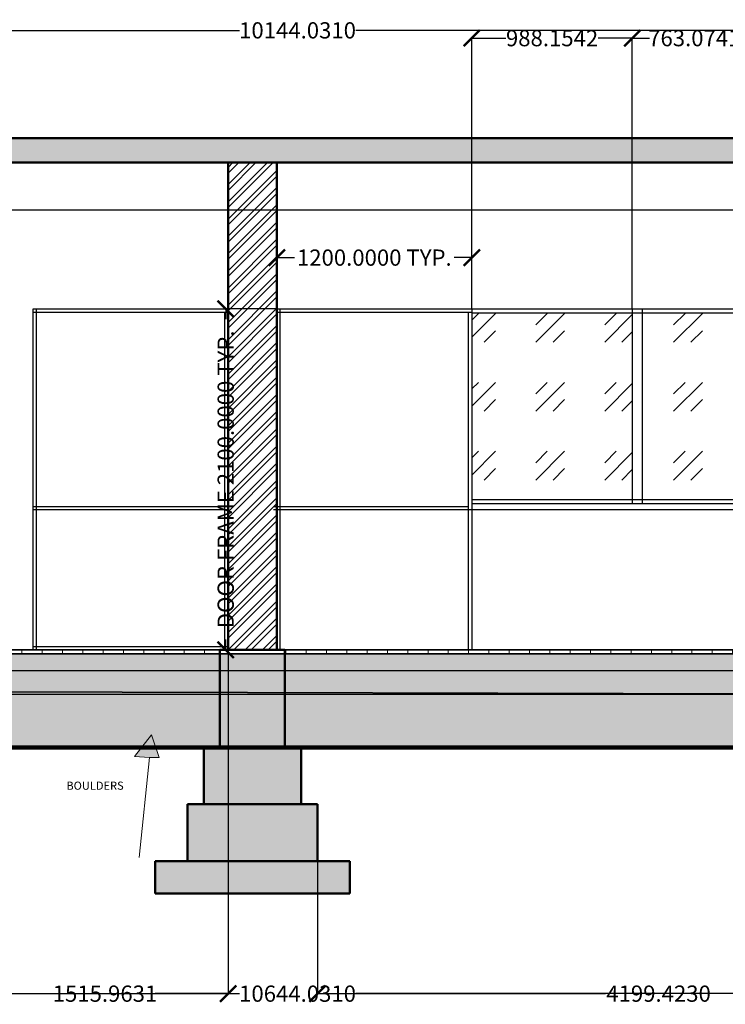
# Model space of a CAD drawing. Units: millimetres. Extents: x -4055 to 12299, y -682 to 5380.
# Tile 2 of 4: x 3612 to 7955, y -682 to 5380. Entities that reach past the tile are written whole.
import ezdxf

# ---------------------------------------------------------------- set-up
doc = ezdxf.new("R2010")
doc.units = ezdxf.units.MM
doc.header["$MEASUREMENT"] = 0
for name, color, linetype, lineweight in [('A-ANNO-DIMS', 2, 'Continuous', 18), ('A-ANNO-SYMB', 18, 'Continuous', 18), ('A-ANNO-TEXT', 7, 'Continuous', 18), ('A-DOOR', 3, 'Continuous', 25), ('A-FLOR', 7, 'Continuous', 35), ('A-FLOR-PATT', 8, 'Continuous', 13), ('A-GLAZ', 4, 'Continuous', 25), ('A-GLAZ-PATT', 8, 'Continuous', 13), ('A-ROOF', 7, 'Continuous', 50), ('A-ROOF-PATT', 8, 'Continuous', 13), ('A-WALL', 7, 'Continuous', 50), ('A-WALL-PATT', 8, 'Continuous', 13), ('gl', 18, 'Continuous', 120), ('S-FNDN', 7, 'Continuous', 50), ('S-FNDN-PATT', 8, 'Continuous', 13)]:
    doc.layers.add(name, color=color, linetype=linetype, lineweight=lineweight)
doc.styles.get("Standard").update_dxf_attribs({"font": 'arial.ttf'})
doc.dimstyles.get("Standard").update_dxf_attribs({"dimtxt": 100, "dimasz": 100, "dimexe": 0.18, "dimexo": 0.0625, "dimgap": 0.09, "dimtad": 0, "dimdec": 4, "dimzin": 0, "dimdsep": 46, "dimtxsty": 'Standard', "dimblk": 'ARCHTICK', "dimcen": 0.09, "dimclrd": 3, "dimclre": 6, "dimclrt": 1, "dimadec": 0, "dimazin": 0, "dimtfac": 1, "dimtdec": 4, "dimtofl": 0, "dimtmove": 0, "dimatfit": 3, "dimfxl": 1, "dimtolj": 1, "dimtzin": 0, "dimlwd": 30, "dimarcsym": 0})
pattern_1 = [(50, (0, 0), (71.72602, -6.2752), [7.5, -82.5]), (355, (0, 0), (-13.87513, 75.2192), [6, -66]), (100.45144, (5.98, -0.52), (57.8509, 68.944), [6.374, -70.1142]), (46.1842, (0, 20), (106.7241, -16.5519), [11.25, -123.75]), (96.6356, (8.89, 18.62), (93.4662, 97.4119), [9.561, -105.1714]), (351.1842, (0, 20), (93.4662, 97.4119), [9, -99]), (21, (10, 15), (59.6907, -40.2619), [7.5, -82.5]), (326, (10, 15), (24.33153, 72.515), [6, -66]), (71.45144, (14.974, 11.645), (84.02224, 32.2531), [6.374, -70.1142]), (37.5, (0, 0), (1.215986, 33.289385), [0, -65.2, 0, -67, 0, -66.25]), (7.5, (0, 0), (26.30695, 39.44117), [0, -38.2, 0, -63.7, 0, -25.25]), (327.5, (-22.3, 0), (53.382244, -2.25549), [0, -25, 0, -78, 0, -103.5]), (317.5, (-32.3, 0), (58.31862, 10.0105), [0, -32.5, 0, -51.8, 0, -73.5])]

# ---------------------------------------------------------------- blocks, each defined once
blk = doc.blocks.new('_ArchTick')
at = {"color": 0, "linetype": 'ByBlock', "const_width": 0.15}
blk.add_lwpolyline([(-0.5, -0.5), (0.5, 0.5)], dxfattribs=at)
blk = doc.blocks.new('*D12')
at = {"layer": 'A-ANNO-DIMS', "color": 0, "lineweight": -2, "transparency": 16777216}
for p, q in [((250, 4650.1), (250, 5314.3)), ((10394, 4650.1), (10394, 5314.3))]:
    blk.add_line(p, q, dxfattribs=at)
at = {"layer": 'A-ANNO-DIMS', "color": 0, "lineweight": 30, "transparency": 16777216}
for p, q in [((250, 5314.1), (4963.8, 5314.1)), ((10394, 5314.1), (5680.2, 5314.1))]:
    blk.add_line(p, q, dxfattribs=at)
at = {"layer": 'Defpoints', "color": 0, "transparency": 16777216}
for p in [(250, 5314.1), (250, 4650), (10394, 4650)]:
    blk.add_point(p, dxfattribs=at)
at = {"layer": 'A-ANNO-DIMS', "color": 0, "lineweight": 30, "transparency": 16777216, "xscale": 100, "yscale": 100, "zscale": 100, "rotation": 180}
blk.add_blockref('_ArchTick', (250, 5314.1), dxfattribs=at)
at = {"layer": 'A-ANNO-DIMS', "color": 0, "lineweight": 30, "transparency": 16777216, "xscale": 100, "yscale": 100, "zscale": 100}
blk.add_blockref('_ArchTick', (10394, 5314.1), dxfattribs=at)
at = {"layer": 'A-ANNO-DIMS', "color": 0, "transparency": 16777216, "insert": (5322, 5314.1), "char_height": 100, "attachment_point": 5}
blk.add_mtext('\\A1;10144.0310', dxfattribs=at)
blk = doc.blocks.new('FNDN-STEPPED-1200')
for p, q in [((-200, 900), (-200, 1500)), ((-200, 1500), (200, 1500)), ((200, 1500), (200, 900)), ((-300, 550), (-300, 900)), ((-300, 900), (300, 900)), ((300, 900), (300, 550)), ((-400, 200), (-400, 550)), ((-400, 550), (400, 550)), ((400, 550), (400, 200)), ((600, 200), (-600, 200)), ((-600, 200), (-600, 0)), ((600, 0), (600, 200)), ((-600, 0), (600, 0))]:
    blk.add_line(p, q)
blk = doc.blocks.new('DOOR-FRAME-1200x2100')
for p, q in [((0, 0), (0, 2100)), ((0, 2100), (1200, 2100)), ((0, 2080), (1200, 2080)), ((20, 0), (20, 2100)), ((1180, 0), (1180, 2080)), ((1200, 0), (0, 0))]:
    blk.add_line(p, q)
blk = doc.blocks.new('NOTE-ARROW')
h = blk.add_hatch(color=256)
h.dxf.hatch_style = 1
h.paths.add_polyline_path([(0, 0), (142, -91.1), (139.1, 2.7), (132.5, 61.8)])
for p, q in [((0, 0), (132.5, 61.8)), ((132.5, 61.8), (139.1, 2.7)), ((758, -0.8), (139.1, 2.7)), ((139.1, 2.7), (142, -91.1)), ((142, -91.1), (0, 0))]:
    blk.add_line(p, q)
blk = doc.blocks.new('*D16')
at = {"layer": 'A-ANNO-DIMS', "color": 6, "lineweight": -2, "transparency": 16777216}
for p, q in [((5194.5, 3600), (4879.4, 3600)), ((5194.5, 1500), (4879.4, 1500))]:
    blk.add_line(p, q, dxfattribs=at)
at = {"layer": 'A-ANNO-DIMS', "color": 3, "lineweight": 30, "transparency": 16777216}
for p, q in [((4879.6, 3600), (4879.6, 3536.3)), ((4879.6, 1500), (4879.6, 1563.7))]:
    blk.add_line(p, q, dxfattribs=at)
at = {"layer": 'Defpoints', "color": 0, "transparency": 16777216}
for p in [(4879.6, 3600), (5194.6, 3600), (5194.6, 1500)]:
    blk.add_point(p, dxfattribs=at)
at = {"layer": 'A-ANNO-DIMS', "color": 3, "lineweight": 30, "transparency": 16777216, "xscale": 100, "yscale": 100, "zscale": 100}
for p, rotation in [((4879.6, 3600), 90), ((4879.6, 1500), 270)]:
    blk.add_blockref('_ArchTick', p, dxfattribs=dict(at, rotation=rotation))
at = {"layer": 'A-ANNO-DIMS', "color": 1, "transparency": 16777216, "insert": (4879.6, 2550), "char_height": 100, "attachment_point": 5, "rotation": 90}
blk.add_mtext('\\A1;DOOR FRAME 2100.0000 TYP.', dxfattribs=at)
blk = doc.blocks.new('*D17')
at = {"layer": 'A-ANNO-DIMS', "color": 6, "lineweight": -2, "transparency": 16777216}
for p, q in [((5194.6, 3600.1), (5194.6, 3915.2)), ((6394.6, 3600.1), (6394.6, 3915.2))]:
    blk.add_line(p, q, dxfattribs=at)
at = {"layer": 'A-ANNO-DIMS', "color": 3, "lineweight": 30, "transparency": 16777216}
for p, q in [((5194.6, 3915), (5303.4, 3915)), ((6394.6, 3915), (6285.9, 3915))]:
    blk.add_line(p, q, dxfattribs=at)
at = {"layer": 'Defpoints', "color": 0, "transparency": 16777216}
for p in [(6394.6, 3915), (5194.6, 3600), (6394.6, 3600)]:
    blk.add_point(p, dxfattribs=at)
at = {"layer": 'A-ANNO-DIMS', "color": 3, "lineweight": 30, "transparency": 16777216, "xscale": 100, "yscale": 100, "zscale": 100, "rotation": 180}
blk.add_blockref('_ArchTick', (5194.6, 3915), dxfattribs=at)
at = {"layer": 'A-ANNO-DIMS', "color": 3, "lineweight": 30, "transparency": 16777216, "xscale": 100, "yscale": 100, "zscale": 100}
blk.add_blockref('_ArchTick', (6394.6, 3915), dxfattribs=at)
at = {"layer": 'A-ANNO-DIMS', "color": 1, "transparency": 16777216, "insert": (5794.6, 3915), "char_height": 100, "attachment_point": 5}
blk.add_mtext('\\A1;1200.0000 TYP.', dxfattribs=at)
blk = doc.blocks.new('*D18')
at = {"layer": 'A-ANNO-DIMS', "color": 6, "lineweight": -2, "transparency": 16777216}
for p, q in [((0, -0.1), (0, -616.4)), ((10644, -0.1), (10644, -616.4))]:
    blk.add_line(p, q, dxfattribs=at)
at = {"layer": 'A-ANNO-DIMS', "color": 3, "lineweight": 30, "transparency": 16777216}
for p, q in [((0, -616.2), (4963.8, -616.2)), ((10644, -616.2), (5680.2, -616.2))]:
    blk.add_line(p, q, dxfattribs=at)
at = {"layer": 'Defpoints', "color": 0, "transparency": 16777216}
for p in [(0, 0), (10644, 0), (10644, -616.2)]:
    blk.add_point(p, dxfattribs=at)
at = {"layer": 'A-ANNO-DIMS', "color": 3, "lineweight": 30, "transparency": 16777216, "xscale": 100, "yscale": 100, "zscale": 100, "rotation": 180}
blk.add_blockref('_ArchTick', (0, -616.2), dxfattribs=at)
at = {"layer": 'A-ANNO-DIMS', "color": 3, "lineweight": 30, "transparency": 16777216, "xscale": 100, "yscale": 100, "zscale": 100}
blk.add_blockref('_ArchTick', (10644, -616.2), dxfattribs=at)
at = {"layer": 'A-ANNO-DIMS', "color": 1, "transparency": 16777216, "insert": (5322, -616.2), "char_height": 100, "attachment_point": 5}
blk.add_mtext('\\A1;10644.0310', dxfattribs=at)
blk = doc.blocks.new('*D20')
at = {"layer": 'A-ANNO-DIMS', "color": 6, "lineweight": -2, "transparency": 16777216}
for p, q in [((3378.6, 4499.9), (3378.6, -616.4)), ((4894.6, 4499.9), (4894.6, -616.4))]:
    blk.add_line(p, q, dxfattribs=at)
at = {"layer": 'A-ANNO-DIMS', "color": 3, "lineweight": 30, "transparency": 16777216}
for p, q in [((3378.6, -616.2), (3826.8, -616.2)), ((4894.6, -616.2), (4446.5, -616.2))]:
    blk.add_line(p, q, dxfattribs=at)
at = {"layer": 'Defpoints', "color": 0, "transparency": 16777216}
for p in [(3378.6, 4500), (4894.6, 4500), (4894.6, -616.2)]:
    blk.add_point(p, dxfattribs=at)
at = {"layer": 'A-ANNO-DIMS', "color": 3, "lineweight": 30, "transparency": 16777216, "xscale": 100, "yscale": 100, "zscale": 100, "rotation": 180}
blk.add_blockref('_ArchTick', (3378.6, -616.2), dxfattribs=at)
at = {"layer": 'A-ANNO-DIMS', "color": 3, "lineweight": 30, "transparency": 16777216, "xscale": 100, "yscale": 100, "zscale": 100}
blk.add_blockref('_ArchTick', (4894.6, -616.2), dxfattribs=at)
at = {"layer": 'A-ANNO-DIMS', "color": 1, "transparency": 16777216, "insert": (4136.6, -616.2), "char_height": 100, "attachment_point": 5}
blk.add_mtext('\\A1;1515.9631', dxfattribs=at)
blk = doc.blocks.new('*D21')
at = {"layer": 'A-ANNO-DIMS', "color": 6, "lineweight": -2, "transparency": 16777216}
for p, q in [((5444.6, 549.9), (5444.6, -616.4)), ((9644, 549.9), (9644, -616.4))]:
    blk.add_line(p, q, dxfattribs=at)
at = {"layer": 'A-ANNO-DIMS', "color": 3, "lineweight": 30, "transparency": 16777216}
for p, q in [((5444.6, -616.2), (7218.3, -616.2)), ((9644, -616.2), (7870.4, -616.2))]:
    blk.add_line(p, q, dxfattribs=at)
at = {"layer": 'Defpoints', "color": 0, "transparency": 16777216}
for p in [(5444.6, 550), (9644, 550), (9644, -616.2)]:
    blk.add_point(p, dxfattribs=at)
at = {"layer": 'A-ANNO-DIMS', "color": 3, "lineweight": 30, "transparency": 16777216, "xscale": 100, "yscale": 100, "zscale": 100, "rotation": 180}
blk.add_blockref('_ArchTick', (5444.6, -616.2), dxfattribs=at)
at = {"layer": 'A-ANNO-DIMS', "color": 3, "lineweight": 30, "transparency": 16777216, "xscale": 100, "yscale": 100, "zscale": 100}
blk.add_blockref('_ArchTick', (9644, -616.2), dxfattribs=at)
at = {"layer": 'A-ANNO-DIMS', "color": 1, "transparency": 16777216, "insert": (7544.3, -616.2), "char_height": 100, "attachment_point": 5}
blk.add_mtext('\\A1;4199.4230', dxfattribs=at)
blk = doc.blocks.new('*D23')
at = {"layer": 'A-ANNO-DIMS', "color": 6, "lineweight": -2, "transparency": 16777216}
for p, q in [((6394.6, 3600.1), (6394.6, 5266.4)), ((7382.8, 3600.1), (7382.8, 5266.4))]:
    blk.add_line(p, q, dxfattribs=at)
at = {"layer": 'A-ANNO-DIMS', "color": 3, "lineweight": 30, "transparency": 16777216}
for p, q in [((6394.6, 5266.2), (6603.8, 5266.2)), ((7382.8, 5266.2), (7173.5, 5266.2))]:
    blk.add_line(p, q, dxfattribs=at)
at = {"layer": 'Defpoints', "color": 0, "transparency": 16777216}
for p in [(7382.8, 5266.2), (6394.6, 3600), (7382.8, 3600)]:
    blk.add_point(p, dxfattribs=at)
at = {"layer": 'A-ANNO-DIMS', "color": 3, "lineweight": 30, "transparency": 16777216, "xscale": 100, "yscale": 100, "zscale": 100, "rotation": 180}
blk.add_blockref('_ArchTick', (6394.6, 5266.2), dxfattribs=at)
at = {"layer": 'A-ANNO-DIMS', "color": 3, "lineweight": 30, "transparency": 16777216, "xscale": 100, "yscale": 100, "zscale": 100}
blk.add_blockref('_ArchTick', (7382.8, 5266.2), dxfattribs=at)
at = {"layer": 'A-ANNO-DIMS', "color": 1, "transparency": 16777216, "insert": (6888.7, 5266.2), "char_height": 100, "attachment_point": 5}
blk.add_mtext('\\A1;988.1542', dxfattribs=at)
blk = doc.blocks.new('*D24')
at = {"layer": 'A-ANNO-DIMS', "color": 6, "lineweight": -2, "transparency": 16777216}
for p, q in [((7382.8, 3600.1), (7382.8, 5266.4)), ((8145.8, 3600.1), (8145.8, 5266.4))]:
    blk.add_line(p, q, dxfattribs=at)
at = {"layer": 'A-ANNO-DIMS', "color": 3, "lineweight": 30, "transparency": 16777216}
for p, q in [((7382.8, 5266.2), (7489, 5266.2)), ((8145.8, 5266.2), (8039.6, 5266.2))]:
    blk.add_line(p, q, dxfattribs=at)
at = {"layer": 'Defpoints', "color": 0, "transparency": 16777216}
for p in [(8145.8, 5266.2), (7382.8, 3600), (8145.8, 3600)]:
    blk.add_point(p, dxfattribs=at)
at = {"layer": 'A-ANNO-DIMS', "color": 3, "lineweight": 30, "transparency": 16777216, "xscale": 100, "yscale": 100, "zscale": 100, "rotation": 180}
blk.add_blockref('_ArchTick', (7382.8, 5266.2), dxfattribs=at)
at = {"layer": 'A-ANNO-DIMS', "color": 3, "lineweight": 30, "transparency": 16777216, "xscale": 100, "yscale": 100, "zscale": 100}
blk.add_blockref('_ArchTick', (8145.8, 5266.2), dxfattribs=at)
at = {"layer": 'A-ANNO-DIMS', "color": 1, "transparency": 16777216, "insert": (7764.3, 5266.2), "char_height": 100, "attachment_point": 5}
blk.add_mtext('\\A1;763.0741', dxfattribs=at)
blk = doc.blocks.new('*D29')
at = {"layer": 'A-ANNO-DIMS', "color": 3, "lineweight": 30, "transparency": 16777216}
for p, q in [((12233, 4500), (12233, 4600)), ((12233, 4209.9), (12233, 4500))]:
    blk.add_line(p, q, dxfattribs=at)
at = {"layer": 'A-ANNO-DIMS', "color": 6, "lineweight": -2, "transparency": 16777216}
for p, q in [((750.1, 4500), (12233.2, 4500)), ((750.1, 4209.9), (12233.2, 4209.9))]:
    blk.add_line(p, q, dxfattribs=at)
at = {"layer": 'Defpoints', "color": 0, "transparency": 16777216}
for p in [(750, 4500), (12233, 4500), (750, 4209.9)]:
    blk.add_point(p, dxfattribs=at)
at = {"layer": 'A-ANNO-DIMS', "color": 3, "lineweight": 30, "transparency": 16777216, "xscale": 100, "yscale": 100, "zscale": 100}
for p, rotation in [((12233, 4500), 90), ((12233, 4209.9), 270)]:
    blk.add_blockref('_ArchTick', p, dxfattribs=dict(at, rotation=rotation))
at = {"layer": 'A-ANNO-DIMS', "color": 1, "transparency": 16777216, "insert": (12233, 4886.2), "char_height": 100, "attachment_point": 5, "rotation": 90}
blk.add_mtext('\\A1;290.1113', dxfattribs=at)
blk = doc.blocks.new('*D31')
at = {"layer": 'A-ANNO-DIMS', "color": 3, "lineweight": 30, "transparency": 16777216}
for p, q in [((-1060.6, 1226), (-1060.6, 1326)), ((-1060.6, 900), (-1060.6, 1226))]:
    blk.add_line(p, q, dxfattribs=at)
at = {"layer": 'A-ANNO-DIMS', "color": 6, "lineweight": -2, "transparency": 16777216}
for p, q in [((9844, 1226), (-1060.8, 1226)), ((9844, 900), (-1060.8, 900))]:
    blk.add_line(p, q, dxfattribs=at)
at = {"layer": 'Defpoints', "color": 0, "transparency": 16777216}
for p in [(-1060.6, 1226), (9844, 1226), (9844, 900)]:
    blk.add_point(p, dxfattribs=at)
at = {"layer": 'A-ANNO-DIMS', "color": 3, "lineweight": 30, "transparency": 16777216, "xscale": 100, "yscale": 100, "zscale": 100}
for p, rotation in [((-1060.6, 1226), 90), ((-1060.6, 900), 270)]:
    blk.add_blockref('_ArchTick', p, dxfattribs=dict(at, rotation=rotation))
at = {"layer": 'A-ANNO-DIMS', "color": 1, "transparency": 16777216, "insert": (-1060.6, 1611.4), "char_height": 100, "attachment_point": 5, "rotation": 90}
blk.add_mtext('\\A1;326.0158', dxfattribs=at)
blk = doc.blocks.new('*D33')
at = {"layer": 'A-ANNO-DIMS', "color": 3, "lineweight": 30, "transparency": 16777216}
for p, q in [((-1060.6, 1500), (-1060.6, 1600)), ((-1060.6, 1370.2), (-1060.6, 1500))]:
    blk.add_line(p, q, dxfattribs=at)
at = {"layer": 'A-ANNO-DIMS', "color": 6, "lineweight": -2, "transparency": 16777216}
for p, q in [((9844, 1500), (-1060.8, 1500)), ((9844, 1370.2), (-1060.8, 1370.2))]:
    blk.add_line(p, q, dxfattribs=at)
at = {"layer": 'Defpoints', "color": 0, "transparency": 16777216}
for p in [(-1060.6, 1500), (9844, 1500), (9844, 1370.2)]:
    blk.add_point(p, dxfattribs=at)
at = {"layer": 'A-ANNO-DIMS', "color": 3, "lineweight": 30, "transparency": 16777216, "xscale": 100, "yscale": 100, "zscale": 100}
for p, rotation in [((-1060.6, 1500), 90), ((-1060.6, 1370.2), 270)]:
    blk.add_blockref('_ArchTick', p, dxfattribs=dict(at, rotation=rotation))
at = {"layer": 'A-ANNO-DIMS', "color": 1, "transparency": 16777216, "insert": (-1060.6, 1871), "char_height": 100, "attachment_point": 5, "rotation": 90}
blk.add_mtext('\\A1;129.7571', dxfattribs=at)
blk = doc.blocks.new('*D34')
at = {"layer": 'A-ANNO-DIMS', "color": 6, "lineweight": -2, "transparency": 16777216}
for p, q in [((6374.7, 2363.8), (12233.2, 2363.8)), ((6374.7, 1500), (12233.2, 1500))]:
    blk.add_line(p, q, dxfattribs=at)
at = {"layer": 'A-ANNO-DIMS', "color": 3, "lineweight": 30, "transparency": 16777216}
for p, q in [((12233, 2363.8), (12233, 2217.3)), ((12233, 1500), (12233, 1646.5))]:
    blk.add_line(p, q, dxfattribs=at)
at = {"layer": 'Defpoints', "color": 0, "transparency": 16777216}
for p in [(6374.6, 2363.8), (12233, 2363.8), (6374.6, 1500)]:
    blk.add_point(p, dxfattribs=at)
at = {"layer": 'A-ANNO-DIMS', "color": 3, "lineweight": 30, "transparency": 16777216, "xscale": 100, "yscale": 100, "zscale": 100}
for p, rotation in [((12233, 2363.8), 90), ((12233, 1500), 270)]:
    blk.add_blockref('_ArchTick', p, dxfattribs=dict(at, rotation=rotation))
at = {"layer": 'A-ANNO-DIMS', "color": 1, "transparency": 16777216, "insert": (12233, 1931.9), "char_height": 100, "attachment_point": 5, "rotation": 90}
blk.add_mtext('\\A1;863.7746', dxfattribs=at)

msp = doc.modelspace()

# ---------------------------------------------------------------- hatches: boundary and pattern name
at = {"layer": 'A-FLOR-PATT'}
h = msp.add_hatch(dxfattribs=at)
h.set_pattern_fill('NET', color=256, scale=1000)
h.paths.add_polyline_path([(3028.64487, 1500), (1878.64487, 1500), (800, 1500), (800, 1475), (3028.64487, 1475)])
h.paths.add_polyline_path([(4844.60797, 1500), (3428.64487, 1500), (3428.64487, 1475), (4844.60797, 1475)])
h.paths.add_polyline_path([(9844.03102, 1500), (5244.60797, 1500), (5244.60797, 1475), (9844.03102, 1475)])
h = msp.add_hatch(dxfattribs=at)
h.set_pattern_fill('AR-SAND', color=256, scale=10)
h.paths.add_polyline_path([(9844.03102, 1475), (5244.60797, 1475), (5244.60797, 1372.3308), (9844.03102, 1370.24292)])
h.paths.add_polyline_path([(4844.60797, 1475), (3428.64487, 1475), (3428.64487, 1373.15514), (4844.60797, 1372.51237)])
h.paths.add_polyline_path([(3428.64487, 1475), (3028.64487, 1475), (3028.64487, 1373.33672), (3428.64487, 1373.15514)])
h.paths.add_polyline_path([(3028.64487, 1475), (800, 1475), (800, 1374.34839), (3028.64487, 1373.33672)])
h = msp.add_hatch(dxfattribs=at)
h.set_pattern_fill('AR-CONC', color=256, scale=10)
h.set_pattern_definition(pattern_1)
h.paths.add_polyline_path([(4844.60797, 1372.51237), (3428.64487, 1373.15514), (3428.64487, 1242.30842), (4844.60797, 1238.71243)])
h.paths.add_polyline_path([(9844.03102, 1370.24292), (5244.60797, 1372.3308), (5244.60797, 1237.69658), (9844.03102, 1226.01584)])
h.paths.add_polyline_path([(3028.64487, 1373.33672), (800, 1374.34839), (800, 1248.98416), (3028.64487, 1243.32427)])
h = msp.add_hatch(dxfattribs=at)
h.set_pattern_fill('GRAVEL', color=256, scale=300)
h.paths.add_polyline_path([(4844.60797, 1238.71243), (3428.64487, 1242.30842), (3428.64487, 900), (4844.60797, 900)])
h.paths.add_polyline_path([(9844.03102, 1226.01584), (5244.60797, 1237.69658), (5244.60797, 900), (9844.03102, 900)])
h.paths.add_polyline_path([(3028.64487, 1243.32427), (800, 1248.98416), (800, 900), (3028.64487, 900)])
at = {"layer": 'A-GLAZ-PATT'}
h = msp.add_hatch(dxfattribs=at)
h.set_pattern_fill('GOST_GLASS', color=256, scale=50)
h.set_pattern_definition([(45, (0, 0), (424.264, 0), [250, -350]), (45, (106.07, 0), (424.264, 0), [100, -500]), (45, (0, 106.07), (424.264, 0), [100, -500])])
h.paths.add_polyline_path([(7382.76217, 3575), (6394.60797, 3575), (6394.60797, 2423.65166), (7382.76163, 2424.08457)])
h.paths.add_polyline_path([(8145.83628, 3575), (7444.13336, 3575), (7444.13282, 2424.11146), (8145.83574, 2424.41887)])
h.paths.add_polyline_path([(8805.9906, 3575), (8207.20748, 3575), (8207.20694, 2424.44576), (8805.99007, 2424.70808)])
h.paths.add_polyline_path([(9410.96289, 3575), (8867.3618, 3575), (8867.36126, 2424.73497), (9410.96235, 2424.97312)])
at = {"layer": 'A-ROOF-PATT'}
h = msp.add_hatch(dxfattribs=at)
h.set_pattern_fill('AR-CONC', color=256, scale=20)
h.set_pattern_definition([(50, (0, 0), (143.452, -12.5504), [15, -165]), (355, (0, 0), (-27.7503, 150.4384), [12, -132]), (100.4514, (11.95, -1.05), (115.7018, 137.888), [12.748, -140.2284]), (46.1842, (0, 40), (213.4483, -33.1039), [22.5, -247.5]), (96.6356, (17.79, 37.24), (186.9324, 194.8237), [19.122, -210.3428]), (351.1842, (0, 40), (186.9324, 194.8237), [18, -198]), (21, (20, 30), (119.3814, -80.5238), [15, -165]), (326, (20, 30), (48.663, 145.03), [12, -132]), (71.4514, (29.95, 23.29), (168.0445, 64.5062), [12.748, -140.2284]), (37.5, (0, 0), (2.43197, 66.57877), [0, -130.4, 0, -134, 0, -132.5]), (7.5, (0, 0), (52.6139, 78.88234), [0, -76.4, 0, -127.4, 0, -50.5]), (327.5, (-44.6, 0), (106.76449, -4.51097), [0, -50, 0, -156, 0, -207]), (317.5, (-64.6, 0), (116.6372, 20.021), [0, -65, 0, -103.6, 0, -147])])
h.paths.add_polyline_path([(10394.03102, 4650), (250, 4650), (250, 4500), (10394.03102, 4500)])
at = {"layer": 'A-WALL-PATT'}
h = msp.add_hatch(dxfattribs=at)
h.set_pattern_fill('ANSI32', color=256, scale=200)
h.paths.add_polyline_path([(750, 3719.22559), (450, 3719.22559), (450, 1500), (750, 1500)])
h.paths.add_polyline_path([(3378.64487, 4500), (3078.64487, 4500), (3078.64487, 1500), (3378.64487, 1500)])
h.paths.add_polyline_path([(5194.60797, 4500), (4894.60797, 4500), (4894.60797, 1500), (5194.60797, 1500), (5194.60797, 3600)])
h.paths.add_polyline_path([(750, 4500), (450, 4500), (450, 4209.88871), (750, 4209.88871)])
h.paths.add_polyline_path([(10194.03102, 4500), (9894.03102, 4500), (9894.03102, 1500), (10194.03102, 1500)])
at = {"layer": 'S-FNDN-PATT'}
h = msp.add_hatch(dxfattribs=at)
h.set_pattern_fill('ANSI33', color=256, scale=400)
h.paths.add_polyline_path([(1000, 550), (200, 550), (200, 200), (1000, 200)])
h.paths.add_polyline_path([(800, 1475), (750, 1475), (400, 1475), (400, 900), (800, 900)])
h.paths.add_polyline_path([(900, 900), (300, 900), (300, 550), (900, 550)])
h.paths.add_polyline_path([(3528.64487, 900), (2928.64487, 900), (2928.64487, 550), (3183.63873, 549.73878), (3186.06833, 624.99556), (3283.2525, 501.18603), (3300.25973, 554.59402), (3528.64487, 550)])
h.paths.add_polyline_path([(3428.64487, 1242.30842), (3028.64487, 1243.32427), (3028.64487, 900), (3428.64487, 900)])
h.paths.add_polyline_path([(3428.64487, 1373.15514), (3028.64487, 1373.33672), (3028.64487, 1243.32427), (3428.64487, 1242.30842)])
h.paths.add_polyline_path([(5244.60797, 1372.3308), (4844.60797, 1372.51237), (4844.60797, 1238.71243), (5244.60797, 1237.69658)])
h.paths.add_polyline_path([(5244.60797, 1237.69658), (4844.60797, 1238.71243), (4844.60797, 900), (5244.60797, 900)])
h.paths.add_polyline_path([(5244.60797, 1475), (4844.60797, 1475), (4844.60797, 1372.51237), (5244.60797, 1372.3308)])
h.paths.add_polyline_path([(5444.60797, 550), (4644.60797, 550), (4644.60797, 200), (5444.60797, 200)])
h.paths.add_polyline_path([(5344.60797, 900), (4744.60797, 900), (4744.60797, 550), (5344.60797, 550)])
h.paths.add_polyline_path([(10344.03102, 900), (9744.03102, 900), (9758.66267, 791.89949), (10329.39937, 791.89949)])
h.paths.add_polyline_path([(10244.03102, 1475), (9894.03102, 1475), (9844.03102, 1475), (9844.03102, 900), (10244.03102, 900)])
h.paths.add_polyline_path([(10444.03102, 550), (9644.03102, 550), (9644.03102, 200), (10444.03102, 200)])
h.paths.add_polyline_path([(9728.20564, 267.06671), (10360.87959, 267.06671), (10329.19473, 421.87571), (9728.20564, 473.13765)], flags=16)
h = msp.add_hatch(dxfattribs=at)
h.set_pattern_fill('AR-CONC', color=256, scale=10)
h.set_pattern_definition(pattern_1)
h.paths.add_polyline_path([(1200, 200), (0, 200), (0, 0), (1200, 0)])
h.paths.add_polyline_path([(5644.60797, 200), (4444.60797, 200), (4444.60797, 0), (5644.60797, 0)])
h.paths.add_polyline_path([(10644.03102, 200), (9444.03102, 200), (9444.03102, 0), (10644.03102, 0)])

# ---------------------------------------------------------------- linework, layer by layer
at = {"layer": 'A-DOOR'}
for p, q in [((6394.60797, 3600), (6394.60797, 1500)), ((3694.60797, 2383.77463), (4894.60797, 2383.77463)), ((5174.60797, 2383.77463), (6374.60797, 2383.77463)), ((3694.60797, 2363.77463), (4894.60797, 2363.77463)), ((5174.60797, 2363.77463), (6374.60797, 2363.77463)), ((3694.60797, 1520), (4894.60797, 1520)), ((3694.60797, 1500), (4894.60797, 1500))]:
    msp.add_line(p, q, dxfattribs=at)
at = {"layer": 'A-FLOR'}
for p, q in [((9894.03102, 1475), (750, 1475)), ((800, 1500), (9844.03102, 1500)), ((800, 1374.34839), (9844.03102, 1370.24292)), ((800, 1248.98416), (9844.03102, 1226.01584))]:
    msp.add_line(p, q, dxfattribs=at)
at = {"layer": 'A-GLAZ'}
for p, q in [((6394.60797, 3600), (9472.33409, 3600)), ((7382.76218, 3600), (7382.76162, 2399.08457)), ((7444.13338, 3600), (7444.13281, 2399.08457)), ((6394.60797, 3575), (9472.33409, 3575)), ((9472.32314, 2425), (6394.59702, 2423.65166)), ((9472.33409, 2400), (6394.60797, 2398.65166))]:
    msp.add_line(p, q, dxfattribs=at)
at = {"layer": 'A-ROOF'}
for p, q in [((10394.03102, 4650), (250, 4650)), ((250, 4500), (10394.03102, 4500))]:
    msp.add_line(p, q, dxfattribs=at)
at = {"layer": 'A-WALL'}
for p, q in [((4894.60797, 1500), (4894.60797, 4500)), ((5194.60797, 4500), (5194.60797, 1500))]:
    msp.add_line(p, q, dxfattribs=at)
at = {"layer": 'gl'}
msp.add_line((800, 900), (9844.03102, 900), dxfattribs=at)

# ---------------------------------------------------------------- block references
at = {"layer": 'A-ANNO-SYMB', "rotation": 264.3956895539121}
msp.add_blockref('NOTE-ARROW', (4422.00115, 976.14262), dxfattribs=at)
at = {"layer": 'A-DOOR'}
for p in [(3694.60797, 1500), (5194.60797, 1500)]:
    msp.add_blockref('DOOR-FRAME-1200x2100', p, dxfattribs=at)
at = {"layer": 'S-FNDN'}
msp.add_blockref('FNDN-STEPPED-1200', (5044.60797, 0), dxfattribs=at)

# ---------------------------------------------------------------- texts
at = {"layer": 'A-ANNO-TEXT', "insert": (3899.04198, 689.09062), "char_height": 50, "attachment_point": 1}
msp.add_mtext_dynamic_manual_height_columns('BOULDERS', width=916.6574754, gutter_width=1, heights=[0], dxfattribs=at)

# ---------------------------------------------------------------- dimensions: what is measured, and where the dimension line sits
at = {"layer": 'A-ANNO-DIMS'}
for base, p1, p2, override, picture, middle in [((250, 5314.10321), (10394.03102, 4650), (250, 4650), {"dimclrd": 0, "dimclre": 0, "dimclrt": 0}, '*D12', (5322.01551, 5314.10321)), ((7382.76218, 5266.25), (6394.60797, 3600), (7382.76218, 3600), {"dimdec": 4, "dimlfac": 1, "dimrnd": 0, "dimzin": 0, "dimdsep": 46, "dimlunit": 2}, '*D23', (6888.68508, 5266.25)), ((8145.8363, 5266.25), (7382.76218, 3600), (8145.8363, 3600), {"dimdec": 4, "dimlfac": 1, "dimrnd": 0, "dimzin": 0, "dimdsep": 46, "dimlunit": 2}, '*D24', (7764.29924, 5266.25)), ((4894.60797, -616.25), (3378.64487, 4500), (4894.60797, 4500), {"dimdec": 4, "dimlfac": 1, "dimrnd": 0, "dimzin": 0, "dimdsep": 46, "dimlunit": 2}, '*D20', (4136.62642, -616.25)), ((9644.031019, -616.25), (5444.607971, 550), (9644.031019, 550), {"dimdec": 4, "dimlfac": 1, "dimrnd": 0, "dimzin": 0, "dimdsep": 46, "dimlunit": 2}, '*D21', (7544.319495, -616.25)), ((10644.03102, -616.25), (0, 0), (10644.03102, 0), {"dimdec": 4, "dimlfac": 1, "dimrnd": 0, "dimzin": 0, "dimdsep": 46, "dimlunit": 2}, '*D18', (5322.01551, -616.25))]:
    dim = msp.add_linear_dim(base=base, p1=p1, p2=p2, dimstyle='Standard', override=override, dxfattribs=at)
    dim.commit()
    dim.dimension.update_dxf_attribs({"geometry": picture, "text_midpoint": middle})
for base, p1, p2, picture, middle in [((12232.99644, 4500), (750, 4209.88871), (750, 4500), '*D29', (12232.99644, 4886.20869)), ((12232.99644, 2363.77463), (6374.60797, 1500), (6374.60797, 2363.77463), '*D34', (12232.99644, 1931.88731)), ((-1060.61411, 1500), (9844.03102, 1370.24292), (9844.03102, 1500), '*D33', (-1060.61411, 1870.99723)), ((-1060.61411, 1226.01584), (9844.03102, 900), (9844.03102, 1226.01584), '*D31', (-1060.61411, 1611.44009))]:
    dim = msp.add_linear_dim(base=base, p1=p1, p2=p2, angle=90, dimstyle='Standard', override={"dimdec": 4, "dimlfac": 1, "dimrnd": 0, "dimzin": 0, "dimdsep": 46, "dimlunit": 2}, dxfattribs=at)
    dim.commit()
    dim.dimension.update_dxf_attribs({"geometry": picture, "text_midpoint": middle})
dim = msp.add_linear_dim(base=(6394.60797, 3915), p1=(5194.60797, 3600), p2=(6394.60797, 3600), text='<> TYP.', dimstyle='Standard', override={"dimdec": 4, "dimlfac": 1, "dimrnd": 0, "dimzin": 0, "dimdsep": 46, "dimlunit": 2}, dxfattribs=at)
dim.commit()
dim.dimension.update_dxf_attribs({"geometry": '*D17', "text_midpoint": (5794.60797, 3915)})
dim = msp.add_linear_dim(base=(4879.60797, 3600), p1=(5194.60797, 1500), p2=(5194.60797, 3600), angle=90, text='DOOR FRAME <> TYP.', dimstyle='Standard', override={"dimdec": 4, "dimlfac": 1, "dimrnd": 0, "dimzin": 0, "dimdsep": 46, "dimlunit": 2}, dxfattribs=at)
dim.commit()
dim.dimension.update_dxf_attribs({"geometry": '*D16', "text_midpoint": (4879.60797, 2550)})

doc.saveas('drawing.dxf')
